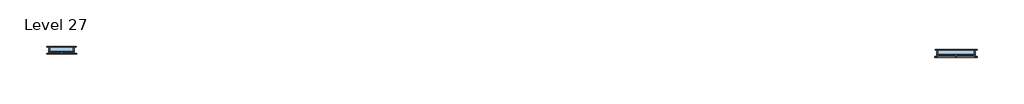
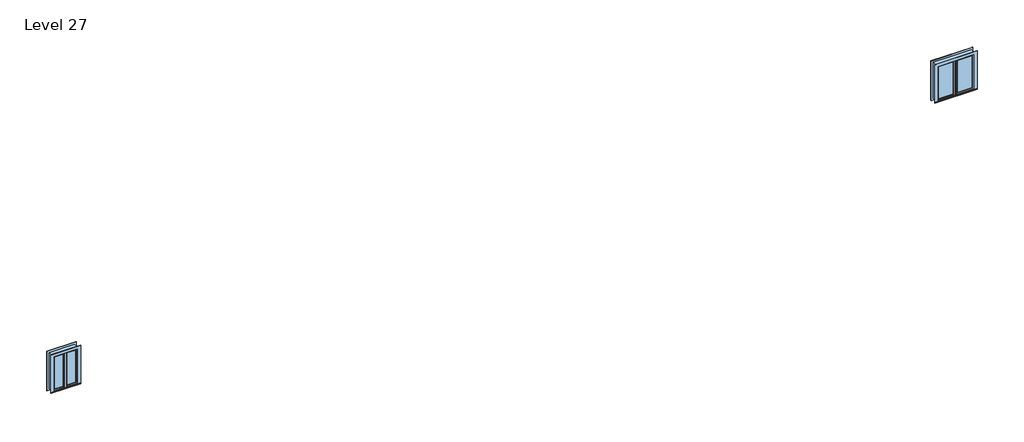
# One storey: 2 windows.
"""IFC4 building model written with IfcOpenShell, lengths in millimetres."""

from ifc_helpers import new_model, si_unit, origin, place, context, project, spatial, transform, mapped, element, save
from components import window_bb17773d, window_0862ab64

model = new_model("IFC4")

# Units and contexts
model_context = context("Model", 3, world=origin())
ifc_project = project(units=[si_unit("LENGTHUNIT", "METRE", prefix="MILLI")], contexts=[model_context])

# Site, building, storey
site = spatial("IfcSite", under=ifc_project)
building = spatial("IfcBuilding", under=site)
storey = spatial("IfcBuildingStorey", under=building, Name="Level 27", Elevation=46329.6)

# Windows
placement = place(None, origin())
window_shape = window_bb17773d(model_context)
element("IfcWindow", 1, ObjectType="Casement Dbl with Trim : 32\" x 48\"", at=placement, inside=storey, context=model_context, shape_type="MappedRepresentation", body=[
    mapped(window_shape, transform((-18502.985279, -12335.6737084, 46329.6), x_axis=(-1.0, 0.0, 0.0), y_axis=(0.0, -1.0, 0.0), z_axis=(0.0, 0.0, 1.0))),
])
window_2_shape = window_0862ab64(model_context)
element("IfcWindow", 2, ObjectType="Casement Dbl with Trim : 48\" x 48\"", at=placement, inside=storey, context=model_context, shape_type="MappedRepresentation", body=[
    mapped(window_2_shape, transform((9924.3594464, -12437.2737084, 46329.6), x_axis=(-1.0, 0.0, 0.0), y_axis=(0.0, -1.0, 0.0), z_axis=(0.0, 0.0, 1.0))),
])

save(model, "model.ifc")

# Revit data of these elements
# Type "Casement Dbl with Trim : 32\" x 48\""
#   Type Mark = "36"
#   Construction Type Id = "GSP4R"
#   Assembly Code = "B2020100"
#   Analytic Construction = "1/8 in Pilkington single glazing"
#   Visual Light Transmittance = 0.9
#   Solar Heat Gain Coefficient = 0.78
#   Heat Transfer Coefficient (U) = 0.6496 BTU/(h·ft²·°F)
#   Height = 4' - 0"
#   Default Sill Height = 3' - 0"
#   Trim Projection - Ext. = 0' - 0 1/2"
#   Trim Projection - Int. = 0' - 0 3/4"
#   Trim Width - Exterior = 0' - 3 1/2"
#   Trim Width - Interior = 0' - 3 1/2"
#   Width = 2' - 8"
#   Window Inset = 0' - 0 3/4"
#   Define Thermal Properties by = 1
#   Glass Pane Material = Glass
#   Sash Material = Sash
#   Trim Exterior Material = Trim
#   Trim Interior Material = Trim
#   Wall Closure = (empty or 0)
# Type "Casement Dbl with Trim : 48\" x 48\""
#   Type Mark = "34"
#   Construction Type Id = "GSP4R"
#   Assembly Code = "B2020100"
#   Analytic Construction = "1/8 in Pilkington single glazing"
#   Visual Light Transmittance = 0.9
#   Solar Heat Gain Coefficient = 0.78
#   Heat Transfer Coefficient (U) = 0.6496 BTU/(h·ft²·°F)
#   Height = 4' - 0"
#   Default Sill Height = 3' - 0"
#   Trim Projection - Ext. = 0' - 0 1/2"
#   Trim Projection - Int. = 0' - 0 3/4"
#   Trim Width - Exterior = 0' - 3 1/2"
#   Trim Width - Interior = 0' - 3 1/2"
#   Width = 4' - 0"
#   Window Inset = 0' - 0 3/4"
#   Define Thermal Properties by = 1
#   Glass Pane Material = Glass
#   Sash Material = Sash
#   Trim Exterior Material = Trim
#   Trim Interior Material = Trim
#   Wall Closure = (empty or 0)
# Element 1 (IfcWindow, "Casement Dbl with Trim : 32\" x 48\"")
#   Mark = "37"
#   Phase Created = New Construction
#   Materials on its faces: "Sash", "Trim", "Glass"
# Element 2 (IfcWindow, "Casement Dbl with Trim : 48\" x 48\"")
#   Mark = "3"
#   Phase Created = New Construction
#   Materials on its faces: "Sash", "Trim", "Glass"
# Materials
#   "Glass": class "Glass", colour RGB 0 128 192, transparency 0.75, Description = "Soda Lime Glass", Cost = 0
#   "Sash": class "Wood", colour RGB 224 178 126, transparency 0
#   "Trim": class "Wood", colour RGB 224 178 126, transparency 0
